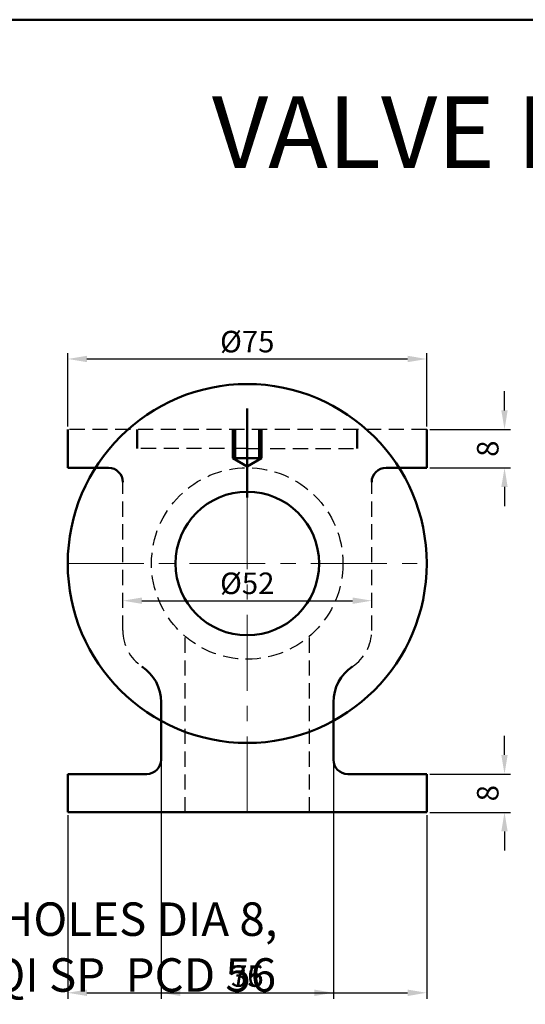
# Model space of a CAD drawing. Units: millimetres. Extents: x -166 to 681, y -4360 to 126.
# Tile 5 of 7: x 153 to 259, y -80 to 126. Entities that reach past the tile are written whole.
import ezdxf
from ezdxf import colors
from ezdxf.entities.mleader import LeaderData, LeaderLine
from ezdxf.math import Vec2, Vec3

# ---------------------------------------------------------------- set-up
doc = ezdxf.new("R2010")
doc.units = ezdxf.units.MM
doc.header["$LTSCALE"] = 0.5
doc.linetypes.add('CENTER', pattern=[50.8, 31.75, -6.35, 6.35, -6.35])
doc.linetypes.add('HIDDEN', pattern=[9.525, 6.35, -3.175])
for name, color, linetype, lineweight in [('M-CNTR', 1, 'CENTER', 18), ('M-DIMS', 2, 'Continuous', 25), ('M-HIDN', 3, 'HIDDEN', 25), ('M-OUTL', 7, 'Continuous', 50), ('M-TEXT', 7, 'Continuous', 25), ('M-TTLB', 7, 'Continuous', 50)]:
    doc.layers.add(name, color=color, linetype=linetype, lineweight=lineweight)
doc.styles.get("Standard").update_dxf_attribs({"font": 'arial.ttf'})
doc.dimstyles.new('ISO-25', dxfattribs={"dimtxt": 4.5, "dimasz": 4, "dimexe": 1.25, "dimexo": 0.625, "dimtad": 1, "dimtoh": 1, "dimdec": 1, "dimtxsty": 'Standard', "dimcen": 2.5, "dimadec": 0, "dimazin": 0, "dimtfac": 1, "dimtdec": 1, "dimtofl": 0, "dimtmove": 0, "dimatfit": 3, "dimfxl": 1, "dimarcsym": 0})

# ---------------------------------------------------------------- blocks, each defined once
blk = doc.blocks.new('*D23')
at = {"layer": 'Defpoints', "color": 0, "ltscale": 0.5, "transparency": 16777216}
for p in [(238.52, 55.18), (163.52, 40.44), (238.52, 40.44)]:
    blk.add_point(p, dxfattribs=at)
at = {"layer": 'M-DIMS', "color": 0, "lineweight": -2, "ltscale": 0.5, "transparency": 16777216}
for p, q in [((163.52, 41.07), (163.52, 56.43)), ((238.52, 41.07), (238.52, 56.43)), ((167.52, 55.18), (234.52, 55.18))]:
    blk.add_line(p, q, dxfattribs=at)
at = {"layer": 'M-DIMS', "color": 0, "ltscale": 0.5, "transparency": 16777216}
for points in [[(167.52, 55.85), (167.52, 54.52), (163.52, 55.18)], [(234.52, 55.85), (234.52, 54.52), (238.52, 55.18)]]:
    blk.add_solid(points, dxfattribs=at)
at = {"layer": 'M-DIMS', "color": 0, "ltscale": 0.5, "transparency": 16777216, "insert": (201.02, 58.23), "char_height": 4.5, "attachment_point": 5}
blk.add_mtext('%%C75', dxfattribs=at)
blk = doc.blocks.new('*D24')
at = {"layer": 'Defpoints', "color": 0, "ltscale": 0.5, "transparency": 16777216}
for p in [(175.02, 4.67), (227.02, 4.67), (227.02, 4.67)]:
    blk.add_point(p, dxfattribs=at)
at = {"layer": 'M-DIMS', "color": 0, "lineweight": -2, "ltscale": 0.5, "transparency": 16777216}
for p, q in [((175.02, 5.3), (175.02, 5.92)), ((179.02, 4.67), (223.02, 4.67)), ((227.02, 5.3), (227.02, 5.92))]:
    blk.add_line(p, q, dxfattribs=at)
at = {"layer": 'M-DIMS', "color": 0, "ltscale": 0.5, "transparency": 16777216}
for points in [[(179.02, 5.34), (179.02, 4), (175.02, 4.67)], [(223.02, 5.34), (223.02, 4), (227.02, 4.67)]]:
    blk.add_solid(points, dxfattribs=at)
at = {"layer": 'M-DIMS', "color": 0, "ltscale": 0.5, "transparency": 16777216, "insert": (201.02, 7.72), "char_height": 4.5, "attachment_point": 5}
blk.add_mtext('%%C52', dxfattribs=at)
blk = doc.blocks.new('*D78')
at = {"layer": 'Defpoints', "color": 0, "ltscale": 0.5, "transparency": 16777216}
for p in [(163.52, -39.56), (238.52, -39.56), (238.52, -77.27)]:
    blk.add_point(p, dxfattribs=at)
at = {"layer": 'M-DIMS', "color": 0, "lineweight": -2, "ltscale": 0.5, "transparency": 16777216}
for p, q in [((163.52, -40.18), (163.52, -78.52)), ((238.52, -40.18), (238.52, -78.52)), ((167.52, -77.27), (234.52, -77.27))]:
    blk.add_line(p, q, dxfattribs=at)
at = {"layer": 'M-DIMS', "color": 0, "ltscale": 0.5, "transparency": 16777216}
for points in [[(167.52, -76.6), (167.52, -77.94), (163.52, -77.27)], [(234.52, -76.6), (234.52, -77.94), (238.52, -77.27)]]:
    blk.add_solid(points, dxfattribs=at)
at = {"layer": 'M-DIMS', "color": 0, "ltscale": 0.5, "transparency": 16777216, "insert": (201.02, -74.36), "char_height": 4.5, "attachment_point": 5}
blk.add_mtext('75', dxfattribs=at)
blk = doc.blocks.new('*D79')
at = {"layer": 'Defpoints', "color": 0, "ltscale": 0.5, "transparency": 16777216}
for p in [(238.52, -31.56), (254.77, -31.56), (238.52, -39.56)]:
    blk.add_point(p, dxfattribs=at)
at = {"layer": 'M-DIMS', "color": 0, "lineweight": -2, "ltscale": 0.5, "transparency": 16777216}
for p, q in [((254.77, -27.56), (254.77, -23.56)), ((239.14, -31.56), (256.02, -31.56)), ((239.14, -39.56), (256.02, -39.56)), ((254.77, -43.56), (254.77, -47.56))]:
    blk.add_line(p, q, dxfattribs=at)
at = {"layer": 'M-DIMS', "color": 0, "ltscale": 0.5, "transparency": 16777216}
for points in [[(254.1, -27.56), (255.43, -27.56), (254.77, -31.56)], [(254.1, -43.56), (255.43, -43.56), (254.77, -39.56)]]:
    blk.add_solid(points, dxfattribs=at)
at = {"layer": 'M-DIMS', "color": 0, "ltscale": 0.5, "transparency": 16777216, "insert": (251.85, -35.56), "char_height": 4.5, "attachment_point": 5, "rotation": 90}
blk.add_mtext('8', dxfattribs=at)
blk = doc.blocks.new('*D80')
at = {"layer": 'Defpoints', "color": 0, "ltscale": 0.5, "transparency": 16777216}
for p in [(238.52, 40.44), (238.52, 32.44), (254.77, 32.44)]:
    blk.add_point(p, dxfattribs=at)
at = {"layer": 'M-DIMS', "color": 0, "lineweight": -2, "ltscale": 0.5, "transparency": 16777216}
for p, q in [((254.77, 44.44), (254.77, 48.44)), ((239.14, 40.44), (256.02, 40.44)), ((239.14, 32.44), (256.02, 32.44)), ((254.77, 28.44), (254.77, 24.44))]:
    blk.add_line(p, q, dxfattribs=at)
at = {"layer": 'M-DIMS', "color": 0, "ltscale": 0.5, "transparency": 16777216}
for points in [[(254.1, 44.44), (255.43, 44.44), (254.77, 40.44)], [(254.1, 28.44), (255.43, 28.44), (254.77, 32.44)]]:
    blk.add_solid(points, dxfattribs=at)
at = {"layer": 'M-DIMS', "color": 0, "ltscale": 0.5, "transparency": 16777216, "insert": (251.85, 36.44), "char_height": 4.5, "attachment_point": 5, "rotation": 90}
blk.add_mtext('8', dxfattribs=at)
blk = doc.blocks.new('*D81')
at = {"layer": 'Defpoints', "color": 0, "ltscale": 0.5, "transparency": 16777216}
for p in [(183.02, -28.56), (219.02, -28.56), (219.02, -77.27)]:
    blk.add_point(p, dxfattribs=at)
at = {"layer": 'M-DIMS', "color": 0, "lineweight": -2, "ltscale": 0.5, "transparency": 16777216}
for p, q in [((183.02, -29.18), (183.02, -78.52)), ((219.02, -29.18), (219.02, -78.52)), ((187.02, -77.27), (215.02, -77.27))]:
    blk.add_line(p, q, dxfattribs=at)
at = {"layer": 'M-DIMS', "color": 0, "ltscale": 0.5, "transparency": 16777216}
for points in [[(187.02, -76.6), (187.02, -77.94), (183.02, -77.27)], [(215.02, -76.6), (215.02, -77.94), (219.02, -77.27)]]:
    blk.add_solid(points, dxfattribs=at)
at = {"layer": 'M-DIMS', "color": 0, "ltscale": 0.5, "transparency": 16777216, "insert": (201.02, -74.35), "char_height": 4.5, "attachment_point": 5}
blk.add_mtext('36', dxfattribs=at)

msp = doc.modelspace()

# ---------------------------------------------------------------- linework, layer by layer
at = {"layer": 'M-CNTR'}
for p, q in [((201.0183, -39.5588), (201.0183, 40.4412)), ((163.5183, 12.4412), (238.5183, 12.4412))]:
    msp.add_line(p, q, dxfattribs=at)
at = {"layer": 'M-HIDN'}
for p, q in [((238.5183, 40.4412), (163.5183, 40.4412)), ((201.0183, 36.4412), (178.0183, 36.4412)), ((201.0183, 36.4412), (224.0183, 36.4412)), ((175.0183, -1.5921), (175.0183, 29.4412)), ((227.0183, -1.5921), (227.0183, 29.4412)), ((188.0183, -39.5588), (188.0183, -2.7574)), ((214.0183, -39.5588), (214.0183, -2.7574))]:
    msp.add_line(p, q, dxfattribs=at)
msp.add_circle((201.0183, 12.4412), 20, dxfattribs=at)
for centre, start, end in [((184.0183, -1.5921), 180, 236.251011), ((218.0183, -1.5921), 303.748989, 0)]:
    msp.add_arc(centre, 9, start, end, dxfattribs=at)
at = {"layer": 'M-OUTL'}
for p, q in [((201.0183, 44.8622), (201.0183, 26.2478)), ((163.5183, 40.4412), (163.5183, 32.4412)), ((178.0183, 36.4412), (178.0183, 40.4412)), ((198.0183, 40.4412), (198.0183, 34.4412)), ((198.5183, 40.4412), (198.5183, 34.1526)), ((203.5183, 40.4412), (203.5183, 34.1526)), ((204.0183, 40.4412), (204.0183, 34.4412)), ((224.0183, 36.4412), (224.0183, 40.4412)), ((238.5183, 32.4412), (238.5183, 40.4412)), ((198.0183, 34.4412), (201.0183, 32.7092)), ((203.5183, 34.4412), (198.5183, 34.4412)), ((201.0183, 32.7092), (204.0183, 34.4412)), ((172.0183, 32.4412), (163.5183, 32.4412)), ((238.5183, 32.4412), (230.0183, 32.4412)), ((183.0183, -28.5588), (183.0183, -16.5588)), ((219.0183, -28.5588), (219.0183, -16.5588)), ((163.5183, -31.5588), (163.5183, -39.5588)), ((163.5183, -31.5588), (180.0183, -31.5588)), ((222.0183, -31.5588), (238.5183, -31.5588)), ((238.5183, -39.5588), (238.5183, -31.5588)), ((163.5183, -39.5588), (238.5183, -39.5588))]:
    msp.add_line(p, q, dxfattribs=at)
for radius in [37.5, 15]:
    msp.add_circle((201.0183, 12.4412), radius, dxfattribs=at)
for centre, radius, start, end in [((172.0183, 29.4412), 3, 0, 90), ((230.0183, 29.4412), 3, 90, 180), ((174.0183, -16.5588), 9, 0, 56.251011), ((228.0183, -16.5588), 9, 123.748989, 180), ((180.0183, -28.5588), 3, 270, 0), ((222.0183, -28.5588), 3, 180, 270)]:
    msp.add_arc(centre, radius, start, end, dxfattribs=at)
at = {"layer": 'M-TTLB', "ltscale": 0.5}
msp.add_lwpolyline([(-165.9437, 126.0872), (680.7907, 126.0872), (680.7907, -430.0081), (-165.9437, -430.0081)], close=True, dxfattribs=at)

# ---------------------------------------------------------------- texts
at = {"layer": 'M-TEXT', "ltscale": 0.5, "insert": (193.6313, 110.0994), "char_height": 15, "attachment_point": 1}
msp.add_mtext_dynamic_manual_height_columns('VALVE MECHANISM', width=215.422355, gutter_width=12.5, heights=[0], dxfattribs=at)

# ---------------------------------------------------------------- dimensions: what is measured, and where the dimension line sits
at = {"layer": 'M-DIMS', "ltscale": 0.5}
for base, p1, p2, picture, middle in [((238.5183, 55.1818), (163.5183, 40.4412), (238.5183, 40.4412), '*D23', (201.0183, 58.2302)), ((227.0183, 4.6703), (175.0183, 4.6703), (227.0183, 4.6703), '*D24', (201.0183, 7.7187))]:
    dim = msp.add_linear_dim(base=base, p1=p1, p2=p2, text='%%C<>', dimstyle='ISO-25', override={"dimclrd": 0, "dimclre": 0, "dimclrt": 0}, dxfattribs=at)
    dim.commit()
    dim.dimension.update_dxf_attribs({"geometry": picture, "text_midpoint": middle})
for base, p1, p2, picture, middle in [((254.7683, 32.4412), (238.5183, 40.4412), (238.5183, 32.4412), '*D80', (251.8457, 36.4412)), ((254.7683, -31.5588), (238.5183, -39.5588), (238.5183, -31.5588), '*D79', (251.8457, -35.5588))]:
    dim = msp.add_linear_dim(base=base, p1=p1, p2=p2, angle=90, dimstyle='ISO-25', override={"dimdec": 0, "dimlfac": 1, "dimrnd": 0, "dimzin": 0, "dimdsep": 46, "dimlunit": 2}, dxfattribs=at)
    dim.commit()
    dim.dimension.update_dxf_attribs({"geometry": picture, "text_midpoint": middle})
for base, p1, p2, picture, middle in [((219.0183, -77.2709), (183.0183, -28.5588), (219.0183, -28.5588), '*D81', (201.0183, -74.3467)), ((238.5183, -77.2709), (163.5183, -39.5588), (238.5183, -39.5588), '*D78', (201.0183, -74.3575))]:
    dim = msp.add_linear_dim(base=base, p1=p1, p2=p2, dimstyle='ISO-25', override={"dimdec": 0, "dimlfac": 1, "dimrnd": 0, "dimzin": 0, "dimdsep": 46, "dimlunit": 2}, dxfattribs=at)
    dim.commit()
    dim.dimension.update_dxf_attribs({"geometry": picture, "text_midpoint": middle})

# ---------------------------------------------------------------- leaders
at = {"layer": 'M-TEXT', "ltscale": 0.5}
ml = msp.add_multileader_mtext('Standard', dxfattribs=at)
ml.set_content('4 HOLES DIA 8,\\P EQI SP  PCD 56', color=256)
ml.set_leader_properties()
ml.build(insert=Vec2(0, 0))
ctx = ml.context
ctx.base_point, ctx.char_height, ctx.plane_origin = Vec3(139.9432, -62.1565), 7, Vec3(114.3904, -39.5588)
notes = []
notes.append((ctx, [(1, (1, 1, 0), (131.9432, -62.1565), (1, 0), 8, [(0, [(114.3904, -39.5588)], 0, [])])]))
ctx.mtext.insert, ctx.mtext.flow_direction = Vec3(141.9432, -58.3843), 5
for ctx, leaders in notes:
    for number, flags, end, landing, length, lines in leaders:
        leader = LeaderData()
        leader.index, (leader.has_last_leader_line, leader.has_dogleg_vector, leader.attachment_direction) = number, flags
        leader.last_leader_point, leader.dogleg_vector, leader.dogleg_length = Vec3(end), Vec3(landing), length
        for number, points, colour, breaks in lines:
            line = LeaderLine()
            line.index, line.vertices, line.color, line.breaks = number, Vec3.list(points), colors.encode_raw_color(colour), breaks
            leader.lines.append(line)
        ctx.leaders.append(leader)

doc.saveas('drawing.dxf')
